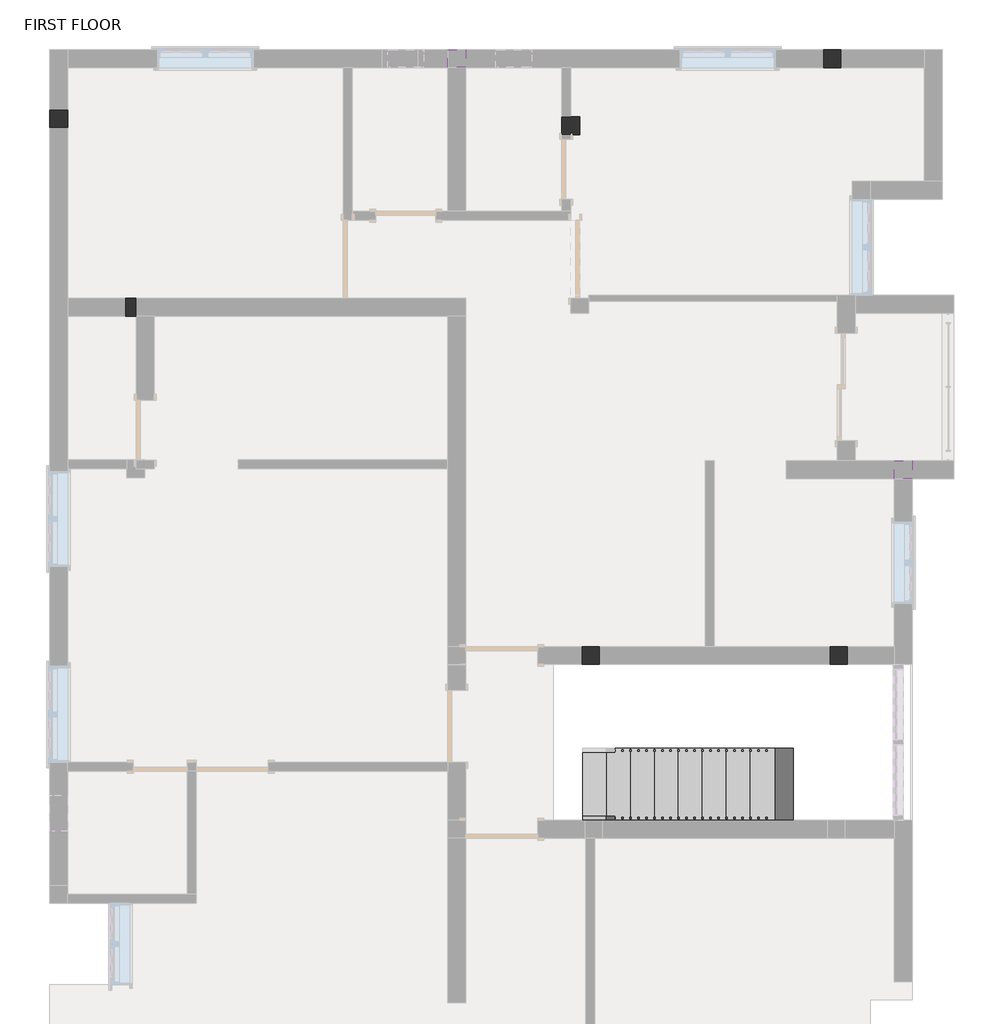
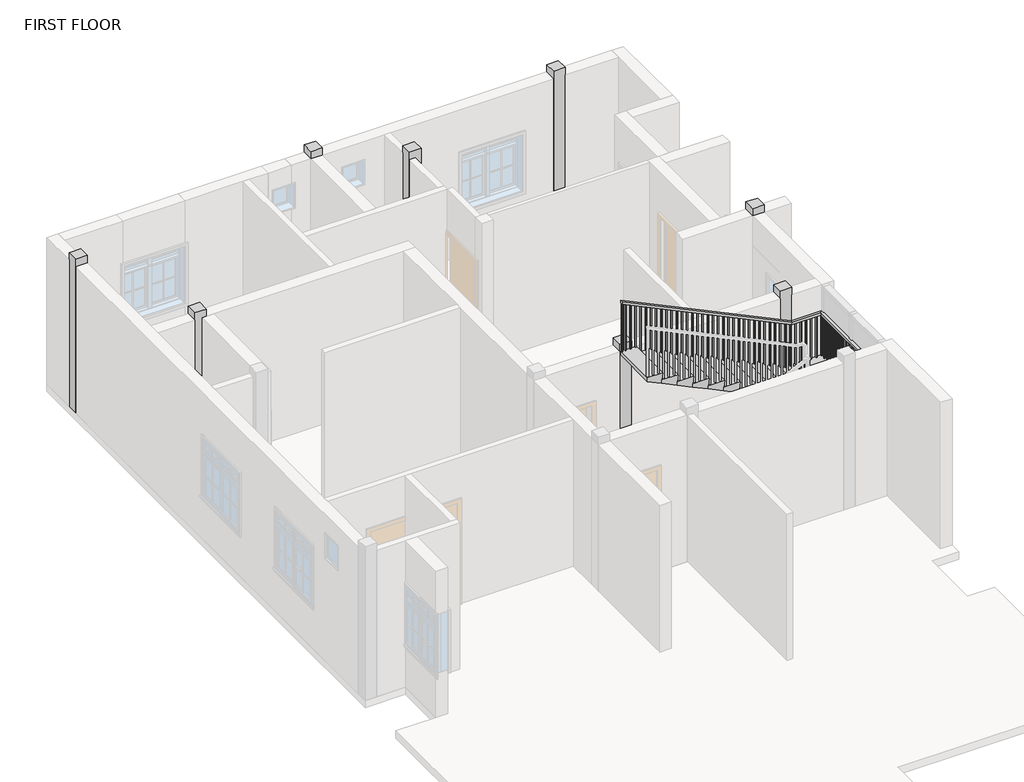
# One storey, part 4 of 6: 8 columns, 1 railing, 1 stair flight.
"""IFC4 building model written with IfcOpenShell, lengths in millimetres."""

from ifc_helpers import new_model, si_unit, frame, origin, place, context, project, spatial, polyline, outline, extrude, faceted_brep, element, save

model = new_model("IFC4")

# Units and contexts
model_context = context("Model", 3, world=origin())
ifc_project = project(units=[si_unit("LENGTHUNIT", "METRE", prefix="MILLI")], contexts=[model_context])

# Site, building, storey
site = spatial("IfcSite", under=ifc_project)
building = spatial("IfcBuilding", under=site)
storey = spatial("IfcBuildingStorey", under=building, Name="FIRST FLOOR", Elevation=3200.4)

# Columns
placement = place(None, origin())
element("IfcColumn", 1, ObjectType="Rectangular Column : 9\"X9\"", at=placement, inside=storey, context=model_context, shape_type="Brep", body=[
    faceted_brep([(-6539.8865981, 8531.2343988, 3200.4), (-6539.8865981, 8302.6343988, 3200.4), (-6768.4865981, 8302.6343988, 3200.4), (-6768.4865981, 8531.2343988, 3200.4), (-6539.8865981, 8531.2343988, 6400.8), (-6539.8865981, 8302.6343988, 6400.8), (-6539.8865981, 8302.6343988, 6248.4), (-6539.8865981, 8531.2343988, 6248.4), (-6768.4865981, 8302.6343988, 6400.8), (-6768.4865981, 8302.6343988, 6248.4), (-6768.4865981, 8531.2343988, 6400.8), (-6768.4865981, 8531.2343988, 6248.4)], [[[0, 1, 2, 3]], [[4, 5, 6, 1, 0, 7]], [[5, 8, 9, 2, 1, 6]], [[8, 10, 11, 3, 2, 9]], [[10, 4, 7, 0, 3, 11]], [[4, 10, 8, 5]]]),
])
element("IfcColumn", 2, ObjectType="Rectangular Column : 9\"X9\"", at=placement, inside=storey, context=model_context, shape_type="Brep", body=[
    faceted_brep([(229.251657, 1705.5787587, 3200.4), (229.251657, 1476.9787587, 3200.4), (0.651657, 1476.9787587, 3200.4), (0.651657, 1705.5787587, 3200.4), (229.251657, 1705.5787587, 6400.8), (229.251657, 1476.9787587, 6400.8), (229.251657, 1476.9787587, 6248.4), (229.251657, 1705.5787587, 6248.4), (0.651657, 1476.9787587, 6400.8), (0.651657, 1476.9787587, 6248.4), (0.651657, 1705.5787587, 6400.8), (0.651657, 1705.5787587, 6248.4)], [[[0, 1, 2, 3]], [[4, 5, 6, 1, 0, 7]], [[5, 8, 9, 2, 1, 6]], [[8, 10, 11, 3, 2, 9]], [[10, 4, 7, 0, 3, 11]], [[4, 10, 8, 5]]]),
])
element("IfcColumn", 3, ObjectType="Rectangular Column : 9\"X9\"", at=placement, inside=storey, context=model_context, shape_type="Brep", body=[
    faceted_brep([(3385.1070369, 1705.5787587, 3200.4), (3385.1070369, 1476.9787587, 3200.4), (3156.5070369, 1476.9787587, 3200.4), (3156.5070369, 1705.5787587, 3200.4), (3385.1070369, 1705.5787587, 6400.8), (3385.1070369, 1476.9787587, 6400.8), (3385.1070369, 1476.9787587, 6248.4), (3385.1070369, 1705.5787587, 6248.4), (3156.5070369, 1476.9787587, 6400.8), (3156.5070369, 1476.9787587, 6248.4), (3156.5070369, 1705.5787587, 6400.8), (3156.5070369, 1705.5787587, 6248.4)], [[[0, 1, 2, 3]], [[4, 5, 6, 1, 0, 7]], [[5, 8, 9, 2, 1, 6]], [[8, 10, 11, 3, 2, 9]], [[10, 4, 7, 0, 3, 11]], [[4, 10, 8, 5]]]),
])
element("IfcColumn", 4, ObjectType="Rectangular Column : 9\"X9\"", at=placement, inside=storey, context=model_context, shape_type="SweptSolid", body=[
    extrude(outline(polyline([(4204.3134019, 4067.7787587), (4204.3134019, 3839.1787587), (3975.7134019, 3839.1787587), (3975.7134019, 4067.7787587), (4204.3134019, 4067.7787587)])), frame((0.0, 0.0, 6248.4), z_axis=(0.0, 0.0, 1.0), x_axis=(1.0, 0.0, 0.0)), (0.0, 0.0, 1.0), 152.4),
])
element("IfcColumn", 5, ObjectType="Rectangular Column : 9\"X9\"", at=placement, inside=storey, context=model_context, shape_type="Brep", body=[
    faceted_brep([(3305.8577655, 9300.1787587, 3200.4), (3305.8577655, 9071.5787587, 3200.4), (3077.2577655, 9071.5787587, 3200.4), (3077.2577655, 9300.1787587, 3200.4), (3305.8577655, 9300.1787587, 6400.8), (3305.8577655, 9071.5787587, 6400.8), (3305.8577655, 9071.5787587, 6248.4), (3305.8577655, 9300.1787587, 6248.4), (3077.2577655, 9071.5787587, 6400.8), (3077.2577655, 9071.5787587, 6248.4), (3077.2577655, 9300.1787587, 6400.8), (3077.2577655, 9300.1787587, 6248.4)], [[[0, 1, 2, 3]], [[4, 5, 6, 1, 0, 7]], [[5, 8, 9, 2, 1, 6]], [[8, 10, 11, 3, 2, 9]], [[10, 4, 7, 0, 3, 11]], [[4, 10, 8, 5]]]),
])
element("IfcColumn", 6, ObjectType="Rectangular Column : 9\"X9\"", at=placement, inside=storey, context=model_context, shape_type="Brep", body=[
    faceted_brep([(-24.7865981, 8443.0921256, 3200.4), (-24.7865981, 8214.4921256, 3200.4), (-139.0865981, 8214.4921256, 3200.4), (-253.3865981, 8214.4921256, 3200.4), (-253.3865981, 8443.0921256, 3200.4), (-139.0865981, 8443.0921256, 3200.4), (-24.7865981, 8443.0921256, 6400.8), (-24.7865981, 8214.4921256, 6400.8), (-253.3865981, 8214.4921256, 6400.8), (-253.3865981, 8214.4921256, 6248.4), (-253.3865981, 8443.0921256, 6400.8), (-253.3865981, 8443.0921256, 6248.4)], [[[0, 1, 2, 3, 4, 5]], [[6, 7, 1, 0]], [[7, 8, 9, 3, 2, 1]], [[8, 10, 11, 4, 3, 9]], [[10, 6, 0, 5, 4, 11]], [[6, 10, 8, 7]]]),
])
element("IfcColumn", 7, ObjectType="Rectangular Column : 9\"X9\"", at=placement, inside=storey, context=model_context, shape_type="Brep", body=[
    faceted_brep([(-5807.056564, 5909.2787587, 3200.4), (-5807.056564, 6137.8787587, 3200.4), (-5663.5865981, 6137.8787587, 3200.4), (-5663.5865981, 5909.2787587, 3200.4), (-5578.456564, 6137.8787587, 6400.8), (-5578.456564, 5909.2787587, 6400.8), (-5578.456564, 5909.2787587, 6248.4), (-5578.456564, 6137.8787587, 6248.4), (-5807.056564, 5909.2787587, 6400.8), (-5807.056564, 5909.2787587, 6248.4), (-5663.5865981, 5909.2787587, 6248.4), (-5807.056564, 6137.8787587, 6400.8), (-5807.056564, 6137.8787587, 6248.4), (-5663.5865981, 6137.8787587, 6248.4)], [[[0, 1, 2, 3]], [[4, 5, 6, 7]], [[5, 8, 9, 0, 3, 10, 6]], [[1, 0, 9, 8, 11, 12]], [[1, 12, 11, 4, 7, 13, 2]], [[5, 4, 11, 8]], [[10, 13, 7, 6]], [[13, 10, 3, 2]]]),
])
element("IfcColumn", 8, ObjectType="Rectangular Column : 9\"X9\"", at=placement, inside=storey, context=model_context, shape_type="SweptSolid", body=[
    extrude(outline(polyline([(-1472.5865981, 9300.1787587), (-1472.5865981, 9071.5787587), (-1701.1865981, 9071.5787587), (-1701.1865981, 9300.1787587), (-1472.5865981, 9300.1787587)])), frame((0.0, 0.0, 6248.4), z_axis=(0.0, 0.0, 1.0), x_axis=(1.0, 0.0, 0.0)), (0.0, 0.0, 1.0), 152.4),
])

# Railing
element("IfcRailing", 9, ObjectType="Handrail - Rectangular", at=placement, inside=storey, context=model_context, shape_type="SolidModel", body=[
    faceted_brep([(13.3134019, -453.4212413, 4260.2727273), (13.3134019, -453.4212413, 4203.9834559), (13.3134019, -504.2212413, 4203.9834559), (13.3134019, -504.2212413, 4260.2727273), (3061.3134019, -453.4212413, 5715.0), (3072.8147322, -453.4212413, 5664.2), (3072.8147322, -504.2212413, 5664.2), (3061.3134019, -504.2212413, 5715.0), (3924.9134019, -453.4212413, 5715.0), (3924.9134019, -453.4212413, 5664.2), (3975.7134019, -504.2212413, 5664.2), (3975.7134019, -504.2212413, 5715.0), (3924.9134019, 1426.1787587, 5715.0), (3924.9134019, 1426.1787587, 5664.2), (3975.7134019, 1476.9787587, 5664.2), (3975.7134019, 1476.9787587, 5715.0), (3366.1134019, 1426.1787587, 5715.0), (3354.6120715, 1426.1787587, 5664.2), (3354.6120715, 1476.9787587, 5664.2), (3366.1134019, 1476.9787587, 5715.0), (13.3134019, 1426.1787587, 7315.2), (13.3134019, 1476.9787587, 7315.2), (13.3134019, 1476.9787587, 7258.9107287), (13.3134019, 1426.1787587, 7258.9107287)], [[[0, 1, 2, 3]], [[1, 0, 4, 5]], [[2, 1, 5, 6]], [[3, 2, 6, 7]], [[0, 3, 7, 4]], [[5, 4, 8, 9]], [[6, 5, 9, 10]], [[7, 6, 10, 11]], [[4, 7, 11, 8]], [[9, 8, 12, 13]], [[10, 9, 13, 14]], [[11, 10, 14, 15]], [[8, 11, 15, 12]], [[13, 12, 16, 17]], [[14, 13, 17, 18]], [[15, 14, 18, 19]], [[12, 15, 19, 16]], [[20, 21, 22, 23]], [[17, 16, 20, 23]], [[18, 17, 23, 22]], [[19, 18, 22, 21]], [[16, 19, 21, 20]]]),
    extrude(outline(polyline([(7217.9965241, 99.0384019), (7227.0885696, 79.9884019), (6255.3272727, 79.9884019), (6255.3272727, 99.0384019), (7217.9965241, 99.0384019)])), frame((0.0, 1442.0537587, 0.0), z_axis=(0.0, 1.0, 0.0), x_axis=(0.0, 0.0, 1.0)), (0.0, 0.0, 1.0), 19.05),
    extrude(outline(polyline([(7169.505615, 200.6384019), (7178.5976605, 181.5884019), (6255.3272727, 181.5884019), (6255.3272727, 200.6384019), (7169.505615, 200.6384019)])), frame((0.0, 1442.0537587, 0.0), z_axis=(0.0, 1.0, 0.0), x_axis=(0.0, 0.0, 1.0)), (0.0, 0.0, 1.0), 19.05),
    extrude(outline(polyline([(7121.0147059, 302.2384019), (7130.1067514, 283.1884019), (6255.3272727, 283.1884019), (6255.3272727, 302.2384019), (7121.0147059, 302.2384019)])), frame((0.0, 1442.0537587, 0.0), z_axis=(0.0, 1.0, 0.0), x_axis=(0.0, 0.0, 1.0)), (0.0, 0.0, 1.0), 19.05),
    extrude(outline(polyline([(7072.5237969, 403.8384019), (7081.6158423, 384.7884019), (6109.8545455, 384.7884019), (6109.8545455, 403.8384019), (7072.5237969, 403.8384019)])), frame((0.0, 1442.0537587, 0.0), z_axis=(0.0, 1.0, 0.0), x_axis=(0.0, 0.0, 1.0)), (0.0, 0.0, 1.0), 19.05),
    extrude(outline(polyline([(7024.0328878, 505.4384019), (7033.1249332, 486.3884019), (6109.8545455, 486.3884019), (6109.8545455, 505.4384019), (7024.0328878, 505.4384019)])), frame((0.0, 1442.0537587, 0.0), z_axis=(0.0, 1.0, 0.0), x_axis=(0.0, 0.0, 1.0)), (0.0, 0.0, 1.0), 19.05),
    extrude(outline(polyline([(6975.5419787, 607.0384019), (6984.6340241, 587.9884019), (6109.8545455, 587.9884019), (6109.8545455, 607.0384019), (6975.5419787, 607.0384019)])), frame((0.0, 1442.0537587, 0.0), z_axis=(0.0, 1.0, 0.0), x_axis=(0.0, 0.0, 1.0)), (0.0, 0.0, 1.0), 19.05),
    extrude(outline(polyline([(6927.0510696, 708.6384019), (6936.143115, 689.5884019), (5964.3818182, 689.5884019), (5964.3818182, 708.6384019), (6927.0510696, 708.6384019)])), frame((0.0, 1442.0537587, 0.0), z_axis=(0.0, 1.0, 0.0), x_axis=(0.0, 0.0, 1.0)), (0.0, 0.0, 1.0), 19.05),
    extrude(outline(polyline([(6878.5601605, 810.2384019), (6887.6522059, 791.1884019), (5964.3818182, 791.1884019), (5964.3818182, 810.2384019), (6878.5601605, 810.2384019)])), frame((0.0, 1442.0537587, 0.0), z_axis=(0.0, 1.0, 0.0), x_axis=(0.0, 0.0, 1.0)), (0.0, 0.0, 1.0), 19.05),
    extrude(outline(polyline([(6830.0692514, 911.8384019), (6839.1612969, 892.7884019), (5964.3818182, 892.7884019), (5964.3818182, 911.8384019), (6830.0692514, 911.8384019)])), frame((0.0, 1442.0537587, 0.0), z_axis=(0.0, 1.0, 0.0), x_axis=(0.0, 0.0, 1.0)), (0.0, 0.0, 1.0), 19.05),
    extrude(outline(polyline([(6781.5783423, 1013.4384019), (6790.6703878, 994.3884019), (5818.9090909, 994.3884019), (5818.9090909, 1013.4384019), (6781.5783423, 1013.4384019)])), frame((0.0, 1442.0537587, 0.0), z_axis=(0.0, 1.0, 0.0), x_axis=(0.0, 0.0, 1.0)), (0.0, 0.0, 1.0), 19.05),
    extrude(outline(polyline([(6733.0874332, 1115.0384019), (6742.1794787, 1095.9884019), (5818.9090909, 1095.9884019), (5818.9090909, 1115.0384019), (6733.0874332, 1115.0384019)])), frame((0.0, 1442.0537587, 0.0), z_axis=(0.0, 1.0, 0.0), x_axis=(0.0, 0.0, 1.0)), (0.0, 0.0, 1.0), 19.05),
    extrude(outline(polyline([(6684.5965241, 1216.6384019), (6693.6885696, 1197.5884019), (5818.9090909, 1197.5884019), (5818.9090909, 1216.6384019), (6684.5965241, 1216.6384019)])), frame((0.0, 1442.0537587, 0.0), z_axis=(0.0, 1.0, 0.0), x_axis=(0.0, 0.0, 1.0)), (0.0, 0.0, 1.0), 19.05),
    extrude(outline(polyline([(6636.105615, 1318.2384019), (6645.1976605, 1299.1884019), (5673.4363636, 1299.1884019), (5673.4363636, 1318.2384019), (6636.105615, 1318.2384019)])), frame((0.0, 1442.0537587, 0.0), z_axis=(0.0, 1.0, 0.0), x_axis=(0.0, 0.0, 1.0)), (0.0, 0.0, 1.0), 19.05),
    extrude(outline(polyline([(6587.6147059, 1419.8384019), (6596.7067514, 1400.7884019), (5673.4363636, 1400.7884019), (5673.4363636, 1419.8384019), (6587.6147059, 1419.8384019)])), frame((0.0, 1442.0537587, 0.0), z_axis=(0.0, 1.0, 0.0), x_axis=(0.0, 0.0, 1.0)), (0.0, 0.0, 1.0), 19.05),
    extrude(outline(polyline([(6539.1237969, 1521.4384019), (6548.2158423, 1502.3884019), (5673.4363636, 1502.3884019), (5673.4363636, 1521.4384019), (6539.1237969, 1521.4384019)])), frame((0.0, 1442.0537587, 0.0), z_axis=(0.0, 1.0, 0.0), x_axis=(0.0, 0.0, 1.0)), (0.0, 0.0, 1.0), 19.05),
    extrude(outline(polyline([(6490.6328878, 1623.0384019), (6499.7249332, 1603.9884019), (5527.9636364, 1603.9884019), (5527.9636364, 1623.0384019), (6490.6328878, 1623.0384019)])), frame((0.0, 1442.0537587, 0.0), z_axis=(0.0, 1.0, 0.0), x_axis=(0.0, 0.0, 1.0)), (0.0, 0.0, 1.0), 19.05),
    extrude(outline(polyline([(6442.1419787, 1724.6384019), (6451.2340241, 1705.5884019), (5527.9636364, 1705.5884019), (5527.9636364, 1724.6384019), (6442.1419787, 1724.6384019)])), frame((0.0, 1442.0537587, 0.0), z_axis=(0.0, 1.0, 0.0), x_axis=(0.0, 0.0, 1.0)), (0.0, 0.0, 1.0), 19.05),
    extrude(outline(polyline([(6393.6510696, 1826.2384019), (6402.743115, 1807.1884019), (5527.9636364, 1807.1884019), (5527.9636364, 1826.2384019), (6393.6510696, 1826.2384019)])), frame((0.0, 1442.0537587, 0.0), z_axis=(0.0, 1.0, 0.0), x_axis=(0.0, 0.0, 1.0)), (0.0, 0.0, 1.0), 19.05),
    extrude(outline(polyline([(6345.1601605, 1927.8384019), (6354.2522059, 1908.7884019), (5382.4909091, 1908.7884019), (5382.4909091, 1927.8384019), (6345.1601605, 1927.8384019)])), frame((0.0, 1442.0537587, 0.0), z_axis=(0.0, 1.0, 0.0), x_axis=(0.0, 0.0, 1.0)), (0.0, 0.0, 1.0), 19.05),
    extrude(outline(polyline([(6296.6692514, 2029.4384019), (6305.7612969, 2010.3884019), (5382.4909091, 2010.3884019), (5382.4909091, 2029.4384019), (6296.6692514, 2029.4384019)])), frame((0.0, 1442.0537587, 0.0), z_axis=(0.0, 1.0, 0.0), x_axis=(0.0, 0.0, 1.0)), (0.0, 0.0, 1.0), 19.05),
    extrude(outline(polyline([(6248.1783423, 2131.0384019), (6257.2703878, 2111.9884019), (5382.4909091, 2111.9884019), (5382.4909091, 2131.0384019), (6248.1783423, 2131.0384019)])), frame((0.0, 1442.0537587, 0.0), z_axis=(0.0, 1.0, 0.0), x_axis=(0.0, 0.0, 1.0)), (0.0, 0.0, 1.0), 19.05),
    extrude(outline(polyline([(6199.6874332, 2232.6384019), (6208.7794787, 2213.5884019), (5237.0181818, 2213.5884019), (5237.0181818, 2232.6384019), (6199.6874332, 2232.6384019)])), frame((0.0, 1442.0537587, 0.0), z_axis=(0.0, 1.0, 0.0), x_axis=(0.0, 0.0, 1.0)), (0.0, 0.0, 1.0), 19.05),
    extrude(outline(polyline([(6151.1965241, 2334.2384019), (6160.2885696, 2315.1884019), (5237.0181818, 2315.1884019), (5237.0181818, 2334.2384019), (6151.1965241, 2334.2384019)])), frame((0.0, 1442.0537587, 0.0), z_axis=(0.0, 1.0, 0.0), x_axis=(0.0, 0.0, 1.0)), (0.0, 0.0, 1.0), 19.05),
    extrude(outline(polyline([(6102.705615, 2435.8384019), (6111.7976605, 2416.7884019), (5237.0181818, 2416.7884019), (5237.0181818, 2435.8384019), (6102.705615, 2435.8384019)])), frame((0.0, 1442.0537587, 0.0), z_axis=(0.0, 1.0, 0.0), x_axis=(0.0, 0.0, 1.0)), (0.0, 0.0, 1.0), 19.05),
    extrude(outline(polyline([(6054.2147059, 2537.4384019), (6063.3067514, 2518.3884019), (5091.5454545, 2518.3884019), (5091.5454545, 2537.4384019), (6054.2147059, 2537.4384019)])), frame((0.0, 1442.0537587, 0.0), z_axis=(0.0, 1.0, 0.0), x_axis=(0.0, 0.0, 1.0)), (0.0, 0.0, 1.0), 19.05),
    extrude(outline(polyline([(6005.7237969, 2639.0384019), (6014.8158423, 2619.9884019), (5091.5454545, 2619.9884019), (5091.5454545, 2639.0384019), (6005.7237969, 2639.0384019)])), frame((0.0, 1442.0537587, 0.0), z_axis=(0.0, 1.0, 0.0), x_axis=(0.0, 0.0, 1.0)), (0.0, 0.0, 1.0), 19.05),
    extrude(outline(polyline([(5957.2328878, 2740.6384019), (5966.3249332, 2721.5884019), (5091.5454545, 2721.5884019), (5091.5454545, 2740.6384019), (5957.2328878, 2740.6384019)])), frame((0.0, 1442.0537587, 0.0), z_axis=(0.0, 1.0, 0.0), x_axis=(0.0, 0.0, 1.0)), (0.0, 0.0, 1.0), 19.05),
    extrude(outline(polyline([(5908.7419787, 2842.2384019), (5917.8340241, 2823.1884019), (4946.0727273, 2823.1884019), (4946.0727273, 2842.2384019), (5908.7419787, 2842.2384019)])), frame((0.0, 1442.0537587, 0.0), z_axis=(0.0, 1.0, 0.0), x_axis=(0.0, 0.0, 1.0)), (0.0, 0.0, 1.0), 19.05),
    extrude(outline(polyline([(5860.2510696, 2943.8384019), (5869.343115, 2924.7884019), (4946.0727273, 2924.7884019), (4946.0727273, 2943.8384019), (5860.2510696, 2943.8384019)])), frame((0.0, 1442.0537587, 0.0), z_axis=(0.0, 1.0, 0.0), x_axis=(0.0, 0.0, 1.0)), (0.0, 0.0, 1.0), 19.05),
    extrude(outline(polyline([(5811.7601605, 3045.4384019), (5820.8522059, 3026.3884019), (4946.0727273, 3026.3884019), (4946.0727273, 3045.4384019), (5811.7601605, 3045.4384019)])), frame((0.0, 1442.0537587, 0.0), z_axis=(0.0, 1.0, 0.0), x_axis=(0.0, 0.0, 1.0)), (0.0, 0.0, 1.0), 19.05),
    extrude(outline(polyline([(5763.2692514, 3147.0384019), (5772.3612969, 3127.9884019), (4800.6, 3127.9884019), (4800.6, 3147.0384019), (5763.2692514, 3147.0384019)])), frame((0.0, 1442.0537587, 0.0), z_axis=(0.0, 1.0, 0.0), x_axis=(0.0, 0.0, 1.0)), (0.0, 0.0, 1.0), 19.05),
    extrude(outline(polyline([(5714.7783423, 3248.6384019), (5723.8703878, 3229.5884019), (4800.6, 3229.5884019), (4800.6, 3248.6384019), (5714.7783423, 3248.6384019)])), frame((0.0, 1442.0537587, 0.0), z_axis=(0.0, 1.0, 0.0), x_axis=(0.0, 0.0, 1.0)), (0.0, 0.0, 1.0), 19.05),
    extrude(outline(polyline([(5666.2874332, 3350.2384019), (5675.3794787, 3331.1884019), (4800.6, 3331.1884019), (4800.6, 3350.2384019), (5666.2874332, 3350.2384019)])), frame((0.0, 1442.0537587, 0.0), z_axis=(0.0, 1.0, 0.0), x_axis=(0.0, 0.0, 1.0)), (0.0, 0.0, 1.0), 19.05),
    extrude(outline(polyline([(3451.8384019, 1461.1037587), (3451.8384019, 1442.0537587), (3432.7884019, 1442.0537587), (3432.7884019, 1461.1037587), (3451.8384019, 1461.1037587)])), frame((0.0, 0.0, 4800.6), z_axis=(0.0, 0.0, 1.0), x_axis=(1.0, 0.0, 0.0)), (0.0, 0.0, 1.0), 863.6),
    extrude(outline(polyline([(3553.4384019, 1461.1037587), (3553.4384019, 1442.0537587), (3534.3884019, 1442.0537587), (3534.3884019, 1461.1037587), (3553.4384019, 1461.1037587)])), frame((0.0, 0.0, 4800.6), z_axis=(0.0, 0.0, 1.0), x_axis=(1.0, 0.0, 0.0)), (0.0, 0.0, 1.0), 863.6),
    extrude(outline(polyline([(3655.0384019, 1461.1037587), (3655.0384019, 1442.0537587), (3635.9884019, 1442.0537587), (3635.9884019, 1461.1037587), (3655.0384019, 1461.1037587)])), frame((0.0, 0.0, 4800.6), z_axis=(0.0, 0.0, 1.0), x_axis=(1.0, 0.0, 0.0)), (0.0, 0.0, 1.0), 863.6),
    extrude(outline(polyline([(3756.6384019, 1461.1037587), (3756.6384019, 1442.0537587), (3737.5884019, 1442.0537587), (3737.5884019, 1461.1037587), (3756.6384019, 1461.1037587)])), frame((0.0, 0.0, 4800.6), z_axis=(0.0, 0.0, 1.0), x_axis=(1.0, 0.0, 0.0)), (0.0, 0.0, 1.0), 863.6),
    extrude(outline(polyline([(3858.2384019, 1461.1037587), (3858.2384019, 1442.0537587), (3839.1884019, 1442.0537587), (3839.1884019, 1461.1037587), (3858.2384019, 1461.1037587)])), frame((0.0, 0.0, 4800.6), z_axis=(0.0, 0.0, 1.0), x_axis=(1.0, 0.0, 0.0)), (0.0, 0.0, 1.0), 863.6),
    extrude(outline(polyline([(3959.8384019, 1340.4537587), (3940.7884019, 1340.4537587), (3940.7884019, 1359.5037587), (3959.8384019, 1359.5037587), (3959.8384019, 1340.4537587)])), frame((0.0, 0.0, 4800.6), z_axis=(0.0, 0.0, 1.0), x_axis=(1.0, 0.0, 0.0)), (0.0, 0.0, 1.0), 863.6),
    extrude(outline(polyline([(3959.8384019, 1238.8537587), (3940.7884019, 1238.8537587), (3940.7884019, 1257.9037587), (3959.8384019, 1257.9037587), (3959.8384019, 1238.8537587)])), frame((0.0, 0.0, 4800.6), z_axis=(0.0, 0.0, 1.0), x_axis=(1.0, 0.0, 0.0)), (0.0, 0.0, 1.0), 863.6),
    extrude(outline(polyline([(3959.8384019, 1137.2537587), (3940.7884019, 1137.2537587), (3940.7884019, 1156.3037587), (3959.8384019, 1156.3037587), (3959.8384019, 1137.2537587)])), frame((0.0, 0.0, 4800.6), z_axis=(0.0, 0.0, 1.0), x_axis=(1.0, 0.0, 0.0)), (0.0, 0.0, 1.0), 863.6),
    extrude(outline(polyline([(3959.8384019, 1035.6537587), (3940.7884019, 1035.6537587), (3940.7884019, 1054.7037587), (3959.8384019, 1054.7037587), (3959.8384019, 1035.6537587)])), frame((0.0, 0.0, 4800.6), z_axis=(0.0, 0.0, 1.0), x_axis=(1.0, 0.0, 0.0)), (0.0, 0.0, 1.0), 863.6),
    extrude(outline(polyline([(3959.8384019, 934.0537587), (3940.7884019, 934.0537587), (3940.7884019, 953.1037587), (3959.8384019, 953.1037587), (3959.8384019, 934.0537587)])), frame((0.0, 0.0, 4800.6), z_axis=(0.0, 0.0, 1.0), x_axis=(1.0, 0.0, 0.0)), (0.0, 0.0, 1.0), 863.6),
    extrude(outline(polyline([(3959.8384019, 832.4537587), (3940.7884019, 832.4537587), (3940.7884019, 851.5037587), (3959.8384019, 851.5037587), (3959.8384019, 832.4537587)])), frame((0.0, 0.0, 4800.6), z_axis=(0.0, 0.0, 1.0), x_axis=(1.0, 0.0, 0.0)), (0.0, 0.0, 1.0), 863.6),
    extrude(outline(polyline([(3959.8384019, 730.8537587), (3940.7884019, 730.8537587), (3940.7884019, 749.9037587), (3959.8384019, 749.9037587), (3959.8384019, 730.8537587)])), frame((0.0, 0.0, 4800.6), z_axis=(0.0, 0.0, 1.0), x_axis=(1.0, 0.0, 0.0)), (0.0, 0.0, 1.0), 863.6),
    extrude(outline(polyline([(3959.8384019, 629.2537587), (3940.7884019, 629.2537587), (3940.7884019, 648.3037587), (3959.8384019, 648.3037587), (3959.8384019, 629.2537587)])), frame((0.0, 0.0, 4800.6), z_axis=(0.0, 0.0, 1.0), x_axis=(1.0, 0.0, 0.0)), (0.0, 0.0, 1.0), 863.6),
    extrude(outline(polyline([(3959.8384019, 527.6537587), (3940.7884019, 527.6537587), (3940.7884019, 546.7037587), (3959.8384019, 546.7037587), (3959.8384019, 527.6537587)])), frame((0.0, 0.0, 4800.6), z_axis=(0.0, 0.0, 1.0), x_axis=(1.0, 0.0, 0.0)), (0.0, 0.0, 1.0), 863.6),
    extrude(outline(polyline([(3959.8384019, 426.0537587), (3940.7884019, 426.0537587), (3940.7884019, 445.1037587), (3959.8384019, 445.1037587), (3959.8384019, 426.0537587)])), frame((0.0, 0.0, 4800.6), z_axis=(0.0, 0.0, 1.0), x_axis=(1.0, 0.0, 0.0)), (0.0, 0.0, 1.0), 863.6),
    extrude(outline(polyline([(3959.8384019, 324.4537587), (3940.7884019, 324.4537587), (3940.7884019, 343.5037587), (3959.8384019, 343.5037587), (3959.8384019, 324.4537587)])), frame((0.0, 0.0, 4800.6), z_axis=(0.0, 0.0, 1.0), x_axis=(1.0, 0.0, 0.0)), (0.0, 0.0, 1.0), 863.6),
    extrude(outline(polyline([(3959.8384019, 222.8537587), (3940.7884019, 222.8537587), (3940.7884019, 241.9037587), (3959.8384019, 241.9037587), (3959.8384019, 222.8537587)])), frame((0.0, 0.0, 4800.6), z_axis=(0.0, 0.0, 1.0), x_axis=(1.0, 0.0, 0.0)), (0.0, 0.0, 1.0), 863.6),
    extrude(outline(polyline([(3959.8384019, 121.2537587), (3940.7884019, 121.2537587), (3940.7884019, 140.3037587), (3959.8384019, 140.3037587), (3959.8384019, 121.2537587)])), frame((0.0, 0.0, 4800.6), z_axis=(0.0, 0.0, 1.0), x_axis=(1.0, 0.0, 0.0)), (0.0, 0.0, 1.0), 863.6),
    extrude(outline(polyline([(3959.8384019, 19.6537587), (3940.7884019, 19.6537587), (3940.7884019, 38.7037587), (3959.8384019, 38.7037587), (3959.8384019, 19.6537587)])), frame((0.0, 0.0, 4800.6), z_axis=(0.0, 0.0, 1.0), x_axis=(1.0, 0.0, 0.0)), (0.0, 0.0, 1.0), 863.6),
    extrude(outline(polyline([(3959.8384019, -81.9462413), (3940.7884019, -81.9462413), (3940.7884019, -62.8962413), (3959.8384019, -62.8962413), (3959.8384019, -81.9462413)])), frame((0.0, 0.0, 4800.6), z_axis=(0.0, 0.0, 1.0), x_axis=(1.0, 0.0, 0.0)), (0.0, 0.0, 1.0), 863.6),
    extrude(outline(polyline([(3959.8384019, -183.5462413), (3940.7884019, -183.5462413), (3940.7884019, -164.4962413), (3959.8384019, -164.4962413), (3959.8384019, -183.5462413)])), frame((0.0, 0.0, 4800.6), z_axis=(0.0, 0.0, 1.0), x_axis=(1.0, 0.0, 0.0)), (0.0, 0.0, 1.0), 863.6),
    extrude(outline(polyline([(3959.8384019, -285.1462413), (3940.7884019, -285.1462413), (3940.7884019, -266.0962413), (3959.8384019, -266.0962413), (3959.8384019, -285.1462413)])), frame((0.0, 0.0, 4800.6), z_axis=(0.0, 0.0, 1.0), x_axis=(1.0, 0.0, 0.0)), (0.0, 0.0, 1.0), 863.6),
    extrude(outline(polyline([(3959.8384019, -386.7462413), (3940.7884019, -386.7462413), (3940.7884019, -367.6962413), (3959.8384019, -367.6962413), (3959.8384019, -386.7462413)])), frame((0.0, 0.0, 4800.6), z_axis=(0.0, 0.0, 1.0), x_axis=(1.0, 0.0, 0.0)), (0.0, 0.0, 1.0), 863.6),
    extrude(outline(polyline([(3864.5884019, -488.3462413), (3864.5884019, -469.2962413), (3883.6384019, -469.2962413), (3883.6384019, -488.3462413), (3864.5884019, -488.3462413)])), frame((0.0, 0.0, 4800.6), z_axis=(0.0, 0.0, 1.0), x_axis=(1.0, 0.0, 0.0)), (0.0, 0.0, 1.0), 863.6),
    extrude(outline(polyline([(3762.9884019, -488.3462413), (3762.9884019, -469.2962413), (3782.0384019, -469.2962413), (3782.0384019, -488.3462413), (3762.9884019, -488.3462413)])), frame((0.0, 0.0, 4800.6), z_axis=(0.0, 0.0, 1.0), x_axis=(1.0, 0.0, 0.0)), (0.0, 0.0, 1.0), 863.6),
    extrude(outline(polyline([(3661.3884019, -488.3462413), (3661.3884019, -469.2962413), (3680.4384019, -469.2962413), (3680.4384019, -488.3462413), (3661.3884019, -488.3462413)])), frame((0.0, 0.0, 4800.6), z_axis=(0.0, 0.0, 1.0), x_axis=(1.0, 0.0, 0.0)), (0.0, 0.0, 1.0), 863.6),
    extrude(outline(polyline([(3559.7884019, -488.3462413), (3559.7884019, -469.2962413), (3578.8384019, -469.2962413), (3578.8384019, -488.3462413), (3559.7884019, -488.3462413)])), frame((0.0, 0.0, 4800.6), z_axis=(0.0, 0.0, 1.0), x_axis=(1.0, 0.0, 0.0)), (0.0, 0.0, 1.0), 863.6),
    extrude(outline(polyline([(3458.1884019, -488.3462413), (3458.1884019, -469.2962413), (3477.2384019, -469.2962413), (3477.2384019, -488.3462413), (3458.1884019, -488.3462413)])), frame((0.0, 0.0, 4800.6), z_axis=(0.0, 0.0, 1.0), x_axis=(1.0, 0.0, 0.0)), (0.0, 0.0, 1.0), 863.6),
    extrude(outline(polyline([(3356.5884019, -488.3462413), (3356.5884019, -469.2962413), (3375.6384019, -469.2962413), (3375.6384019, -488.3462413), (3356.5884019, -488.3462413)])), frame((0.0, 0.0, 4800.6), z_axis=(0.0, 0.0, 1.0), x_axis=(1.0, 0.0, 0.0)), (0.0, 0.0, 1.0), 863.6),
    extrude(outline(polyline([(3254.9884019, -488.3462413), (3254.9884019, -469.2962413), (3274.0384019, -469.2962413), (3274.0384019, -488.3462413), (3254.9884019, -488.3462413)])), frame((0.0, 0.0, 4800.6), z_axis=(0.0, 0.0, 1.0), x_axis=(1.0, 0.0, 0.0)), (0.0, 0.0, 1.0), 863.6),
    extrude(outline(polyline([(3153.3884019, -488.3462413), (3153.3884019, -469.2962413), (3172.4384019, -469.2962413), (3172.4384019, -488.3462413), (3153.3884019, -488.3462413)])), frame((0.0, 0.0, 4800.6), z_axis=(0.0, 0.0, 1.0), x_axis=(1.0, 0.0, 0.0)), (0.0, 0.0, 1.0), 863.6),
    extrude(outline(polyline([(5663.2567514, 3070.8384019), (5654.1647059, 3051.7884019), (4800.6, 3051.7884019), (4800.6, 3070.8384019), (5663.2567514, 3070.8384019)])), frame((0.0, -488.3462413, 0.0), z_axis=(0.0, 1.0, 0.0), x_axis=(0.0, 0.0, 1.0)), (0.0, 0.0, 1.0), 19.05),
    extrude(outline(polyline([(5614.7658423, 2969.2384019), (5605.6737969, 2950.1884019), (4655.1272727, 2950.1884019), (4655.1272727, 2969.2384019), (5614.7658423, 2969.2384019)])), frame((0.0, -488.3462413, 0.0), z_axis=(0.0, 1.0, 0.0), x_axis=(0.0, 0.0, 1.0)), (0.0, 0.0, 1.0), 19.05),
    extrude(outline(polyline([(5566.2749332, 2867.6384019), (5557.1828878, 2848.5884019), (4655.1272727, 2848.5884019), (4655.1272727, 2867.6384019), (5566.2749332, 2867.6384019)])), frame((0.0, -488.3462413, 0.0), z_axis=(0.0, 1.0, 0.0), x_axis=(0.0, 0.0, 1.0)), (0.0, 0.0, 1.0), 19.05),
    extrude(outline(polyline([(5517.7840241, 2766.0384019), (5508.6919787, 2746.9884019), (4655.1272727, 2746.9884019), (4655.1272727, 2766.0384019), (5517.7840241, 2766.0384019)])), frame((0.0, -488.3462413, 0.0), z_axis=(0.0, 1.0, 0.0), x_axis=(0.0, 0.0, 1.0)), (0.0, 0.0, 1.0), 19.05),
    extrude(outline(polyline([(5469.293115, 2664.4384019), (5460.2010696, 2645.3884019), (4509.6545455, 2645.3884019), (4509.6545455, 2664.4384019), (5469.293115, 2664.4384019)])), frame((0.0, -488.3462413, 0.0), z_axis=(0.0, 1.0, 0.0), x_axis=(0.0, 0.0, 1.0)), (0.0, 0.0, 1.0), 19.05),
    extrude(outline(polyline([(5420.8022059, 2562.8384019), (5411.7101605, 2543.7884019), (4509.6545455, 2543.7884019), (4509.6545455, 2562.8384019), (5420.8022059, 2562.8384019)])), frame((0.0, -488.3462413, 0.0), z_axis=(0.0, 1.0, 0.0), x_axis=(0.0, 0.0, 1.0)), (0.0, 0.0, 1.0), 19.05),
    extrude(outline(polyline([(5372.3112969, 2461.2384019), (5363.2192514, 2442.1884019), (4509.6545455, 2442.1884019), (4509.6545455, 2461.2384019), (5372.3112969, 2461.2384019)])), frame((0.0, -488.3462413, 0.0), z_axis=(0.0, 1.0, 0.0), x_axis=(0.0, 0.0, 1.0)), (0.0, 0.0, 1.0), 19.05),
    extrude(outline(polyline([(5323.8203878, 2359.6384019), (5314.7283423, 2340.5884019), (4364.1818182, 2340.5884019), (4364.1818182, 2359.6384019), (5323.8203878, 2359.6384019)])), frame((0.0, -488.3462413, 0.0), z_axis=(0.0, 1.0, 0.0), x_axis=(0.0, 0.0, 1.0)), (0.0, 0.0, 1.0), 19.05),
    extrude(outline(polyline([(5275.3294787, 2258.0384019), (5266.2374332, 2238.9884019), (4364.1818182, 2238.9884019), (4364.1818182, 2258.0384019), (5275.3294787, 2258.0384019)])), frame((0.0, -488.3462413, 0.0), z_axis=(0.0, 1.0, 0.0), x_axis=(0.0, 0.0, 1.0)), (0.0, 0.0, 1.0), 19.05),
    extrude(outline(polyline([(5226.8385696, 2156.4384019), (5217.7465241, 2137.3884019), (4364.1818182, 2137.3884019), (4364.1818182, 2156.4384019), (5226.8385696, 2156.4384019)])), frame((0.0, -488.3462413, 0.0), z_axis=(0.0, 1.0, 0.0), x_axis=(0.0, 0.0, 1.0)), (0.0, 0.0, 1.0), 19.05),
    extrude(outline(polyline([(5178.3476605, 2054.8384019), (5169.255615, 2035.7884019), (4218.7090909, 2035.7884019), (4218.7090909, 2054.8384019), (5178.3476605, 2054.8384019)])), frame((0.0, -488.3462413, 0.0), z_axis=(0.0, 1.0, 0.0), x_axis=(0.0, 0.0, 1.0)), (0.0, 0.0, 1.0), 19.05),
    extrude(outline(polyline([(5129.8567514, 1953.2384019), (5120.7647059, 1934.1884019), (4218.7090909, 1934.1884019), (4218.7090909, 1953.2384019), (5129.8567514, 1953.2384019)])), frame((0.0, -488.3462413, 0.0), z_axis=(0.0, 1.0, 0.0), x_axis=(0.0, 0.0, 1.0)), (0.0, 0.0, 1.0), 19.05),
    extrude(outline(polyline([(5081.3658423, 1851.6384019), (5072.2737969, 1832.5884019), (4218.7090909, 1832.5884019), (4218.7090909, 1851.6384019), (5081.3658423, 1851.6384019)])), frame((0.0, -488.3462413, 0.0), z_axis=(0.0, 1.0, 0.0), x_axis=(0.0, 0.0, 1.0)), (0.0, 0.0, 1.0), 19.05),
    extrude(outline(polyline([(5032.8749332, 1750.0384019), (5023.7828878, 1730.9884019), (4073.2363636, 1730.9884019), (4073.2363636, 1750.0384019), (5032.8749332, 1750.0384019)])), frame((0.0, -488.3462413, 0.0), z_axis=(0.0, 1.0, 0.0), x_axis=(0.0, 0.0, 1.0)), (0.0, 0.0, 1.0), 19.05),
    extrude(outline(polyline([(4984.3840241, 1648.4384019), (4975.2919787, 1629.3884019), (4073.2363636, 1629.3884019), (4073.2363636, 1648.4384019), (4984.3840241, 1648.4384019)])), frame((0.0, -488.3462413, 0.0), z_axis=(0.0, 1.0, 0.0), x_axis=(0.0, 0.0, 1.0)), (0.0, 0.0, 1.0), 19.05),
    extrude(outline(polyline([(4935.893115, 1546.8384019), (4926.8010696, 1527.7884019), (4073.2363636, 1527.7884019), (4073.2363636, 1546.8384019), (4935.893115, 1546.8384019)])), frame((0.0, -488.3462413, 0.0), z_axis=(0.0, 1.0, 0.0), x_axis=(0.0, 0.0, 1.0)), (0.0, 0.0, 1.0), 19.05),
    extrude(outline(polyline([(4887.4022059, 1445.2384019), (4878.3101605, 1426.1884019), (3927.7636364, 1426.1884019), (3927.7636364, 1445.2384019), (4887.4022059, 1445.2384019)])), frame((0.0, -488.3462413, 0.0), z_axis=(0.0, 1.0, 0.0), x_axis=(0.0, 0.0, 1.0)), (0.0, 0.0, 1.0), 19.05),
    extrude(outline(polyline([(4838.9112969, 1343.6384019), (4829.8192514, 1324.5884019), (3927.7636364, 1324.5884019), (3927.7636364, 1343.6384019), (4838.9112969, 1343.6384019)])), frame((0.0, -488.3462413, 0.0), z_axis=(0.0, 1.0, 0.0), x_axis=(0.0, 0.0, 1.0)), (0.0, 0.0, 1.0), 19.05),
    extrude(outline(polyline([(4790.4203878, 1242.0384019), (4781.3283423, 1222.9884019), (3927.7636364, 1222.9884019), (3927.7636364, 1242.0384019), (4790.4203878, 1242.0384019)])), frame((0.0, -488.3462413, 0.0), z_axis=(0.0, 1.0, 0.0), x_axis=(0.0, 0.0, 1.0)), (0.0, 0.0, 1.0), 19.05),
    extrude(outline(polyline([(4741.9294787, 1140.4384019), (4732.8374332, 1121.3884019), (3782.2909091, 1121.3884019), (3782.2909091, 1140.4384019), (4741.9294787, 1140.4384019)])), frame((0.0, -488.3462413, 0.0), z_axis=(0.0, 1.0, 0.0), x_axis=(0.0, 0.0, 1.0)), (0.0, 0.0, 1.0), 19.05),
    extrude(outline(polyline([(4693.4385696, 1038.8384019), (4684.3465241, 1019.7884019), (3782.2909091, 1019.7884019), (3782.2909091, 1038.8384019), (4693.4385696, 1038.8384019)])), frame((0.0, -488.3462413, 0.0), z_axis=(0.0, 1.0, 0.0), x_axis=(0.0, 0.0, 1.0)), (0.0, 0.0, 1.0), 19.05),
    extrude(outline(polyline([(4644.9476605, 937.2384019), (4635.855615, 918.1884019), (3782.2909091, 918.1884019), (3782.2909091, 937.2384019), (4644.9476605, 937.2384019)])), frame((0.0, -488.3462413, 0.0), z_axis=(0.0, 1.0, 0.0), x_axis=(0.0, 0.0, 1.0)), (0.0, 0.0, 1.0), 19.05),
    extrude(outline(polyline([(4596.4567514, 835.6384019), (4587.3647059, 816.5884019), (3636.8181818, 816.5884019), (3636.8181818, 835.6384019), (4596.4567514, 835.6384019)])), frame((0.0, -488.3462413, 0.0), z_axis=(0.0, 1.0, 0.0), x_axis=(0.0, 0.0, 1.0)), (0.0, 0.0, 1.0), 19.05),
    extrude(outline(polyline([(4547.9658423, 734.0384019), (4538.8737969, 714.9884019), (3636.8181818, 714.9884019), (3636.8181818, 734.0384019), (4547.9658423, 734.0384019)])), frame((0.0, -488.3462413, 0.0), z_axis=(0.0, 1.0, 0.0), x_axis=(0.0, 0.0, 1.0)), (0.0, 0.0, 1.0), 19.05),
    extrude(outline(polyline([(4499.4749332, 632.4384019), (4490.3828878, 613.3884019), (3636.8181818, 613.3884019), (3636.8181818, 632.4384019), (4499.4749332, 632.4384019)])), frame((0.0, -488.3462413, 0.0), z_axis=(0.0, 1.0, 0.0), x_axis=(0.0, 0.0, 1.0)), (0.0, 0.0, 1.0), 19.05),
    extrude(outline(polyline([(4450.9840241, 530.8384019), (4441.8919787, 511.7884019), (3491.3454545, 511.7884019), (3491.3454545, 530.8384019), (4450.9840241, 530.8384019)])), frame((0.0, -488.3462413, 0.0), z_axis=(0.0, 1.0, 0.0), x_axis=(0.0, 0.0, 1.0)), (0.0, 0.0, 1.0), 19.05),
    extrude(outline(polyline([(4402.493115, 429.2384019), (4393.4010696, 410.1884019), (3491.3454545, 410.1884019), (3491.3454545, 429.2384019), (4402.493115, 429.2384019)])), frame((0.0, -488.3462413, 0.0), z_axis=(0.0, 1.0, 0.0), x_axis=(0.0, 0.0, 1.0)), (0.0, 0.0, 1.0), 19.05),
    extrude(outline(polyline([(4354.0022059, 327.6384019), (4344.9101605, 308.5884019), (3491.3454545, 308.5884019), (3491.3454545, 327.6384019), (4354.0022059, 327.6384019)])), frame((0.0, -488.3462413, 0.0), z_axis=(0.0, 1.0, 0.0), x_axis=(0.0, 0.0, 1.0)), (0.0, 0.0, 1.0), 19.05),
    extrude(outline(polyline([(4305.5112969, 226.0384019), (4296.4192514, 206.9884019), (3345.8727273, 206.9884019), (3345.8727273, 226.0384019), (4305.5112969, 226.0384019)])), frame((0.0, -488.3462413, 0.0), z_axis=(0.0, 1.0, 0.0), x_axis=(0.0, 0.0, 1.0)), (0.0, 0.0, 1.0), 19.05),
    extrude(outline(polyline([(4257.0203878, 124.4384019), (4247.9283423, 105.3884019), (3345.8727273, 105.3884019), (3345.8727273, 124.4384019), (4257.0203878, 124.4384019)])), frame((0.0, -488.3462413, 0.0), z_axis=(0.0, 1.0, 0.0), x_axis=(0.0, 0.0, 1.0)), (0.0, 0.0, 1.0), 19.05),
    extrude(outline(polyline([(3959.8384019, 1442.0537587), (3940.7884019, 1442.0537587), (3940.7884019, 1461.1037587), (3959.8384019, 1461.1037587), (3959.8384019, 1442.0537587)])), frame((0.0, 0.0, 4800.6), z_axis=(0.0, 0.0, 1.0), x_axis=(1.0, 0.0, 0.0)), (0.0, 0.0, 1.0), 863.6),
    extrude(outline(polyline([(3940.7884019, -488.3462413), (3940.7884019, -469.2962413), (3959.8384019, -469.2962413), (3959.8384019, -488.3462413), (3940.7884019, -488.3462413)])), frame((0.0, 0.0, 4800.6), z_axis=(0.0, 0.0, 1.0), x_axis=(1.0, 0.0, 0.0)), (0.0, 0.0, 1.0), 863.6),
    extrude(outline(polyline([(7249.8186832, 32.3634019), (7258.9107287, 13.3134019), (6255.3272727, 13.3134019), (6255.3272727, 32.3634019), (7249.8186832, 32.3634019)])), frame((0.0, 1442.0537587, 0.0), z_axis=(0.0, 1.0, 0.0), x_axis=(0.0, 0.0, 1.0)), (0.0, 0.0, 1.0), 19.05),
    extrude(outline(polyline([(4213.0755014, 32.3634019), (4203.9834559, 13.3134019), (3345.8727273, 13.3134019), (3345.8727273, 32.3634019), (4213.0755014, 32.3634019)])), frame((0.0, -488.3462413, 0.0), z_axis=(0.0, 1.0, 0.0), x_axis=(0.0, 0.0, 1.0)), (0.0, 0.0, 1.0), 19.05),
])

# Stair flight
element("IfcStairFlight", 10, ObjectType="3/4\" Nosing", at=placement, inside=storey, context=model_context, shape_type="Brep", body=[
    faceted_brep([(13.3134019, 410.1787587, 3345.8727273), (13.3134019, -504.2212413, 3345.8727273), (337.1634019, -504.2212413, 3345.8727273), (337.1634019, 410.1787587, 3345.8727273), (337.1634019, 410.1787587, 3275.5111381), (179.7876839, 410.1787587, 3200.4), (32.3634019, 410.1787587, 3200.4), (32.3634019, -504.2212413, 3200.4), (179.7876839, -504.2212413, 3200.4), (337.1634019, -504.2212413, 3275.5111381), (318.1134019, 410.1787587, 3491.3454545), (318.1134019, -504.2212413, 3491.3454545), (641.9634019, -504.2212413, 3491.3454545), (641.9634019, 410.1787587, 3491.3454545), (641.9634019, 410.1787587, 3420.9838654), (641.9634019, -504.2212413, 3420.9838654), (622.9134019, 410.1787587, 3636.8181818), (622.9134019, -504.2212413, 3636.8181818), (946.7634019, -504.2212413, 3636.8181818), (946.7634019, 410.1787587, 3636.8181818), (946.7634019, 410.1787587, 3566.4565927), (946.7634019, -504.2212413, 3566.4565927), (927.7134019, 410.1787587, 3782.2909091), (927.7134019, -504.2212413, 3782.2909091), (1251.5634019, -504.2212413, 3782.2909091), (1251.5634019, 410.1787587, 3782.2909091), (1251.5634019, 410.1787587, 3711.9293199), (1251.5634019, -504.2212413, 3711.9293199), (1232.5134019, 410.1787587, 3927.7636364), (1232.5134019, -504.2212413, 3927.7636364), (1556.3634019, -504.2212413, 3927.7636364), (1556.3634019, 410.1787587, 3927.7636364), (1556.3634019, 410.1787587, 3857.4020472), (1556.3634019, -504.2212413, 3857.4020472), (1537.3134019, 410.1787587, 4073.2363636), (1537.3134019, -504.2212413, 4073.2363636), (1861.1634019, -504.2212413, 4073.2363636), (1861.1634019, 410.1787587, 4073.2363636), (1861.1634019, 410.1787587, 4002.8747745), (1861.1634019, -504.2212413, 4002.8747745), (1842.1134019, 410.1787587, 4218.7090909), (1842.1134019, -504.2212413, 4218.7090909), (2165.9634019, -504.2212413, 4218.7090909), (2165.9634019, 410.1787587, 4218.7090909), (2165.9634019, 410.1787587, 4148.3475018), (2165.9634019, -504.2212413, 4148.3475018), (2146.9134019, 410.1787587, 4364.1818182), (2146.9134019, -504.2212413, 4364.1818182), (2470.7634019, -504.2212413, 4364.1818182), (2470.7634019, 410.1787587, 4364.1818182), (2470.7634019, 410.1787587, 4293.820229), (2470.7634019, -504.2212413, 4293.820229), (2451.7134019, 410.1787587, 4509.6545455), (2451.7134019, -504.2212413, 4509.6545455), (2775.5634019, -504.2212413, 4509.6545455), (2775.5634019, 410.1787587, 4509.6545455), (2775.5634019, 410.1787587, 4439.2929563), (2775.5634019, -504.2212413, 4439.2929563), (3080.3634019, 410.1787587, 4655.1272727), (2756.5134019, 410.1787587, 4655.1272727), (2756.5134019, -504.2212413, 4655.1272727), (3080.3634019, -504.2212413, 4655.1272727), (3069.628878, 410.1787587, 4737.1), (3399.5400648, 410.1787587, 4737.1), (3080.3634019, -504.2212413, 4584.7656836), (3042.2634019, 562.5787587, 4800.6), (3061.3134019, 562.5787587, 4800.6), (3061.3134019, 410.1787587, 4800.6), (3061.3134019, -504.2212413, 4800.6), (3399.5400648, -504.2212413, 4800.6), (3975.7134019, -504.2212413, 4800.6), (3975.7134019, 1476.9787587, 4800.6), (3042.2634019, 1476.9787587, 4800.6), (3042.2634019, 562.5787587, 4737.1), (3061.3134019, 562.5787587, 4737.1), (3061.3134019, 410.1787587, 4737.1), (3399.5400648, -504.2212413, 4737.1), (3975.7134019, -504.2212413, 4737.1), (3975.7134019, 1476.9787587, 4737.1), (3042.2634019, 1476.9787587, 4737.1), (3061.3134019, 562.5787587, 4946.0727273), (3061.3134019, 1476.9787587, 4946.0727273), (3027.8867389, 1476.9787587, 4946.0727273), (2737.4634019, 1476.9787587, 4946.0727273), (2737.4634019, 562.5787587, 4946.0727273), (3027.8867389, 562.5787587, 4946.0727273), (2737.4634019, 562.5787587, 4875.7111381), (3027.8867389, 562.5787587, 4737.1), (3027.8867389, 1476.9787587, 4737.1), (2737.4634019, 1476.9787587, 4875.7111381), (2756.5134019, 562.5787587, 5091.5454545), (2756.5134019, 1476.9787587, 5091.5454545), (2432.6634019, 1476.9787587, 5091.5454545), (2432.6634019, 562.5787587, 5091.5454545), (2432.6634019, 562.5787587, 5021.1838654), (2432.6634019, 1476.9787587, 5021.1838654), (2451.7134019, 562.5787587, 5237.0181818), (2451.7134019, 1476.9787587, 5237.0181818), (2127.8634019, 1476.9787587, 5237.0181818), (2127.8634019, 562.5787587, 5237.0181818), (2127.8634019, 562.5787587, 5166.6565927), (2127.8634019, 1476.9787587, 5166.6565927), (2146.9134019, 562.5787587, 5382.4909091), (2146.9134019, 1476.9787587, 5382.4909091), (1823.0634019, 1476.9787587, 5382.4909091), (1823.0634019, 562.5787587, 5382.4909091), (1823.0634019, 562.5787587, 5312.1293199), (1823.0634019, 1476.9787587, 5312.1293199), (1842.1134019, 562.5787587, 5527.9636364), (1842.1134019, 1476.9787587, 5527.9636364), (1518.2634019, 1476.9787587, 5527.9636364), (1518.2634019, 562.5787587, 5527.9636364), (1518.2634019, 562.5787587, 5457.6020472), (1518.2634019, 1476.9787587, 5457.6020472), (1537.3134019, 562.5787587, 5673.4363636), (1537.3134019, 1476.9787587, 5673.4363636), (1213.4634019, 1476.9787587, 5673.4363636), (1213.4634019, 562.5787587, 5673.4363636), (1213.4634019, 562.5787587, 5603.0747745), (1213.4634019, 1476.9787587, 5603.0747745), (1232.5134019, 562.5787587, 5818.9090909), (1232.5134019, 1476.9787587, 5818.9090909), (908.6634019, 1476.9787587, 5818.9090909), (908.6634019, 562.5787587, 5818.9090909), (908.6634019, 562.5787587, 5748.5475018), (908.6634019, 1476.9787587, 5748.5475018), (927.7134019, 562.5787587, 5964.3818182), (927.7134019, 1476.9787587, 5964.3818182), (603.8634019, 1476.9787587, 5964.3818182), (603.8634019, 562.5787587, 5964.3818182), (603.8634019, 562.5787587, 5894.020229), (603.8634019, 1476.9787587, 5894.020229), (622.9134019, 562.5787587, 6109.8545455), (622.9134019, 1476.9787587, 6109.8545455), (299.0634019, 1476.9787587, 6109.8545455), (299.0634019, 562.5787587, 6109.8545455), (299.0634019, 562.5787587, 6039.4929563), (299.0634019, 1476.9787587, 6039.4929563), (318.1134019, 562.5787587, 6255.3272727), (318.1134019, 1476.9787587, 6255.3272727), (13.3134019, 1476.9787587, 6255.3272727), (13.3134019, 562.5787587, 6255.3272727), (13.3134019, 562.5787587, 6175.8736381), (13.3134019, 1476.9787587, 6175.8736381)], [[[0, 1, 2, 3]], [[0, 3, 4, 5, 6]], [[2, 1, 7, 8, 9]], [[10, 11, 12, 13]], [[10, 13, 14, 4, 3]], [[12, 11, 2, 9, 15]], [[16, 17, 18, 19]], [[16, 19, 20, 14, 13]], [[18, 17, 12, 15, 21]], [[22, 23, 24, 25]], [[22, 25, 26, 20, 19]], [[24, 23, 18, 21, 27]], [[28, 29, 30, 31]], [[28, 31, 32, 26, 25]], [[30, 29, 24, 27, 33]], [[34, 35, 36, 37]], [[34, 37, 38, 32, 31]], [[36, 35, 30, 33, 39]], [[40, 41, 42, 43]], [[40, 43, 44, 38, 37]], [[42, 41, 36, 39, 45]], [[46, 47, 48, 49]], [[46, 49, 50, 44, 43]], [[48, 47, 42, 45, 51]], [[52, 53, 54, 55]], [[52, 55, 56, 50, 49]], [[54, 53, 48, 51, 57]], [[58, 59, 60, 61]], [[58, 62, 63, 56, 55, 59]], [[61, 60, 54, 57, 64]], [[65, 66, 67, 68, 69, 70, 71, 72]], [[66, 65, 73, 74]], [[67, 66, 74, 75]], [[62, 67, 75]], [[68, 61, 64, 76, 77, 70, 69]], [[71, 70, 77, 78]], [[72, 71, 78, 79]], [[80, 81, 82, 83, 84, 85]], [[65, 80, 85, 84, 86, 87, 73]], [[81, 72, 79, 88, 89, 83, 82]], [[90, 91, 92, 93]], [[90, 93, 94, 86, 84]], [[92, 91, 83, 89, 95]], [[96, 97, 98, 99]], [[96, 99, 100, 94, 93]], [[98, 97, 92, 95, 101]], [[102, 103, 104, 105]], [[102, 105, 106, 100, 99]], [[104, 103, 98, 101, 107]], [[108, 109, 110, 111]], [[108, 111, 112, 106, 105]], [[110, 109, 104, 107, 113]], [[114, 115, 116, 117]], [[114, 117, 118, 112, 111]], [[116, 115, 110, 113, 119]], [[120, 121, 122, 123]], [[120, 123, 124, 118, 117]], [[122, 121, 116, 119, 125]], [[126, 127, 128, 129]], [[126, 129, 130, 124, 123]], [[128, 127, 122, 125, 131]], [[132, 133, 134, 135]], [[132, 135, 136, 130, 129]], [[134, 133, 128, 131, 137]], [[1, 0, 6, 7]], [[3, 2, 11, 10]], [[13, 12, 17, 16]], [[19, 18, 23, 22]], [[25, 24, 29, 28]], [[31, 30, 35, 34]], [[37, 36, 41, 40]], [[43, 42, 47, 46]], [[49, 48, 53, 52]], [[55, 54, 60, 59]], [[58, 61, 68, 67, 62]], [[65, 72, 81, 80]], [[84, 83, 91, 90]], [[93, 92, 97, 96]], [[99, 98, 103, 102]], [[105, 104, 109, 108]], [[111, 110, 115, 114]], [[117, 116, 121, 120]], [[123, 122, 127, 126]], [[129, 128, 133, 132]], [[138, 139, 140, 141]], [[138, 141, 142, 136, 135]], [[140, 139, 134, 137, 143]], [[141, 140, 143, 142]], [[135, 134, 139, 138]], [[7, 6, 5, 8]], [[56, 63, 76, 64, 57, 51, 45, 39, 33, 27, 21, 15, 9, 8, 5, 4, 14, 20, 26, 32, 38, 44, 50]], [[76, 63, 62, 75, 74, 73, 87, 88, 79, 78, 77]], [[88, 87, 86, 94, 100, 106, 112, 118, 124, 130, 136, 142, 143, 137, 131, 125, 119, 113, 107, 101, 95, 89]]]),
])

save(model, "model.ifc")

# Revit data of these elements
# Type "Rectangular Column : 9\"X9\""
#   Assembly Code = "B1010200"
#   Depth = 0' - 9"
#   Offset Base = 0' - 0"
#   Offset Top = 0' - 0"
#   Width = 0' - 9"
#   Material = none
# Type "Handrail - Rectangular"
#   Assembly Code = "C2010400"
#   built-in parameter 1008612 = 0.0416667 (stored number, unit not read)
#   built-in parameter 1008611 = 0.0416667 (stored number, unit not read)
#   built-in parameter 1008609 = 0.333333 (stored number, unit not read)
#   built-in parameter 1008604 = 0.166667 (stored number, unit not read)
#   built-in parameter 1008603 = 0.166667 (stored number, unit not read)
#   Railing Height = 3' - 0"
#   built-in parameter 1008630 = 2
#   built-in parameter 1008610 = 2
#   built-in parameter 1008618 = Baluster - Square : 3/4"
# Elements 1, 2, 3, 4, 7, 8 (IfcColumn, "Rectangular Column : 9\"X9\"")
#   Phase Created = New Construction
#   Materials on its faces: "wall"
# Element 5 (IfcColumn, "Rectangular Column : 9\"X9\"")
#   Phase Created = New Construction
#   Materials on its faces: "wall", "wood"
# Element 6 (IfcColumn, "Rectangular Column : 9\"X9\"")
#   Phase Created = New Construction
#   Materials on its faces: "Default Wall"
# Element 9 (IfcRailing, "Handrail - Rectangular")
#   Phase Created = New Construction
# Element 10 (IfcStairFlight, "3/4\" Nosing")
#   Phase Created = New Construction
#   Materials on its faces: "Concrete, Cast-in-Place gray"
# Materials
#   "wall": class "Generic", colour RGB 112 128 144, transparency 0, Cost = 0
#   "wood": class "Generic", colour RGB 155 131 132, transparency 0, Cost = 0
#   "Default Wall": colour RGB 128 128 128, transparency 0, Cost = 0
#   "Concrete, Cast-in-Place gray": class "Concrete", colour RGB 192 192 192, transparency 0, Description = "Cast-in-place concrete", Cost = 0
